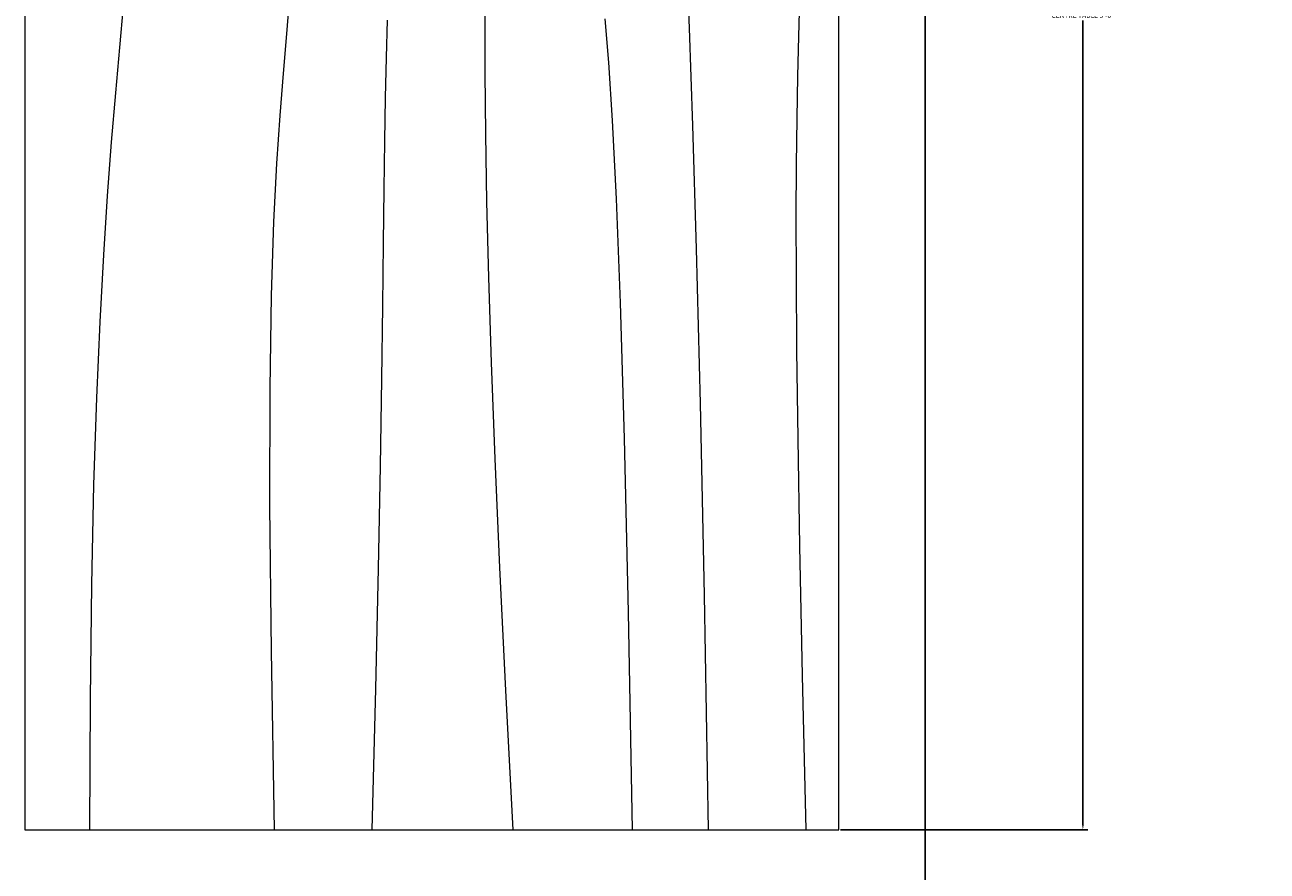
# Model space of a CAD drawing. Units: inches. Extents: x -105 to 1196, y -792 to 119.
# Tile 12 of 23: x 232 to 278, y -380 to -349. Entities that reach past the tile are written whole.
import ezdxf

# ---------------------------------------------------------------- set-up
doc = ezdxf.new("R2010")
doc.units = ezdxf.units.IN
doc.header["$MEASUREMENT"] = 0
doc.layers.add('A-ANNO-DIMS', color=2, linetype='Continuous', lineweight=18)
doc.layers.add('A-FURN', color=8, linetype='Continuous', lineweight=18)
doc.styles.get("Standard").update_dxf_attribs({"font": 'arial.ttf'})
doc.dimstyles.get("Standard").update_dxf_attribs({"dimtxt": 0.18, "dimasz": 0.18, "dimexe": 0.18, "dimexo": 0.0625, "dimgap": 0.09, "dimtad": 0, "dimtih": 1, "dimtoh": 1, "dimdec": 1, "dimzin": 0, "dimdsep": 46, "dimlunit": 4, "dimtxsty": 'Standard', "dimcen": 0.09, "dimadec": 0, "dimazin": 0, "dimtfac": 1, "dimtdec": 1, "dimtofl": 0, "dimtmove": 0, "dimatfit": 3, "dimfxl": 1, "dimtolj": 1, "dimtzin": 0, "dimarcsym": 0})

# ---------------------------------------------------------------- blocks, each defined once
blk = doc.blocks.new('Table - Rectangular Woodgrain 60 x 30 in.')
for p, q in [((0, 0), (0, -30)), ((60, 0), (0, 0)), ((0, -30), (60, -30))]:
    blk.add_line(p, q)
for points in [[(0, -2.4), (4.8155, -2.418), (9.0302, -2.4688), (12.709, -2.5477), (15.9167, -2.65), (18.7181, -2.7711), (21.1781, -2.9063), (23.3616, -3.0508), (25.3333, -3.2), (27.1477, -3.3495), (28.8172, -3.4958), (30.3437, -3.636)], [(0, -9.2), (6.5759, -9.0858), (11.9385, -9.0365), (16.2527, -9.0418), (19.6833, -9.0917), (22.3952, -9.1759), (24.5531, -9.2844), (26.322, -9.4069), (27.8666, -9.5333), (29.3241, -9.6553), (30.7203, -9.7719)], [(0, -12.8), (5.1847, -12.9322), (9.6213, -13.0323), (13.3963, -13.1059), (16.5958, -13.1583), (19.3063, -13.1952), (21.614, -13.2219), (23.6054, -13.2439), (25.3666, -13.2667), (26.9728, -13.2947), (28.4531, -13.3281), (29.8256, -13.3663)], [(0, -18), (5.124, -17.7273), (9.6609, -17.5057), (13.6705, -17.3303), (17.2125, -17.1958), (20.3467, -17.0973), (23.1328, -17.0297), (25.6307, -16.9878), (27.9, -16.9667), (29.9928, -16.9617)], [(0, -22.4), (8.0098, -22.2501), (14.4094, -22.1011), (19.4168, -21.9535), (23.25, -21.8083), (26.1269, -21.6663), (28.2656, -21.5281), (29.884, -21.3947)], [(0, -25.2), (8.6355, -25.0504), (15.7026, -24.9031), (21.4049, -24.7606), (25.9458, -24.625), (29.529, -24.4988), (32.3578, -24.3844)], [(0, -28.8), (5.6867, -28.6681), (10.45, -28.5698), (14.407, -28.5012), (17.675, -28.4584), (20.3711, -28.4374), (22.6125, -28.4344), (24.5164, -28.4455), (26.2, -28.4667), (27.762, -28.4947), (29.2276, -28.5281), (30.6033, -28.5663)]]:
    blk.add_lwpolyline(points)
blk = doc.blocks.new('*D77')
at = {"layer": 'A-ANNO-DIMS', "color": 0, "lineweight": -2, "transparency": 16777216}
for p, q in [((277.544, -304.122), (264.827, -304.122)), ((265.007, -304.302), (265.007, -345.939)), ((265.007, -387.942), (265.007, -346.305)), ((277.544, -388.122), (264.827, -388.122))]:
    blk.add_line(p, q, dxfattribs=at)
at = {"layer": 'A-ANNO-DIMS', "color": 0, "transparency": 16777216}
for points in [[(264.977, -304.302), (265.037, -304.302), (265.007, -304.122)], [(264.977, -387.942), (265.037, -387.942), (265.007, -388.122)]]:
    blk.add_solid(points, dxfattribs=at)
at = {"layer": 'Defpoints', "color": 0, "transparency": 16777216}
for p in [(277.607, -304.122), (265.007, -388.122), (277.607, -388.122)]:
    blk.add_point(p, dxfattribs=at)
at = {"layer": 'A-ANNO-DIMS', "color": 0, "transparency": 16777216, "insert": (265.007, -346.122), "char_height": 0.18, "attachment_point": 5}
blk.add_mtext('\\A1;SOFA 7\'-0"', dxfattribs=at)
blk = doc.blocks.new('*D83')
at = {"layer": 'A-ANNO-DIMS', "color": 0, "lineweight": -2, "transparency": 16777216}
for p, q in [((261.878, -318.695), (270.995, -318.695)), ((270.815, -318.875), (270.815, -348.512)), ((270.815, -378.515), (270.815, -348.878)), ((261.878, -378.695), (270.995, -378.695))]:
    blk.add_line(p, q, dxfattribs=at)
at = {"layer": 'A-ANNO-DIMS', "color": 0, "transparency": 16777216}
for points in [[(270.785, -318.875), (270.845, -318.875), (270.815, -318.695)], [(270.785, -378.515), (270.845, -378.515), (270.815, -378.695)]]:
    blk.add_solid(points, dxfattribs=at)
at = {"layer": 'Defpoints', "color": 0, "transparency": 16777216}
for p in [(261.815, -318.695), (270.815, -318.695), (261.815, -378.695)]:
    blk.add_point(p, dxfattribs=at)
at = {"layer": 'A-ANNO-DIMS', "color": 0, "transparency": 16777216, "insert": (270.815, -348.695), "char_height": 0.18, "attachment_point": 5}
blk.add_mtext('\\A1;CENTRE TABLE 5\'-0"', dxfattribs=at)

msp = doc.modelspace()

# ---------------------------------------------------------------- block references
at = {"layer": 'A-FURN', "rotation": 90}
msp.add_blockref('Table - Rectangular Woodgrain 60 x 30 in.', (231.815, -378.695), dxfattribs=at)

# ---------------------------------------------------------------- dimensions: what is measured, and where the dimension line sits
at = {"layer": 'A-ANNO-DIMS'}
for base, p1, p2, angle, text, picture, middle in [((265.007, -388.122), (277.607, -304.122), (277.607, -388.122), 270, 'SOFA <>', '*D77', (265.007, -346.122)), ((270.815, -318.695), (261.815, -378.695), (261.815, -318.695), 90, 'CENTRE TABLE <>', '*D83', (270.815, -348.695))]:
    dim = msp.add_linear_dim(base=base, p1=p1, p2=p2, angle=angle, text=text, dimstyle='Standard', override={"dimdec": 1, "dimlfac": 1, "dimrnd": 0, "dimzin": 1, "dimdsep": 46, "dimlunit": 4, "dimfrac": 2}, dxfattribs=at)
    dim.commit()
    dim.dimension.update_dxf_attribs({"geometry": picture, "text_midpoint": middle})

doc.saveas('drawing.dxf')
